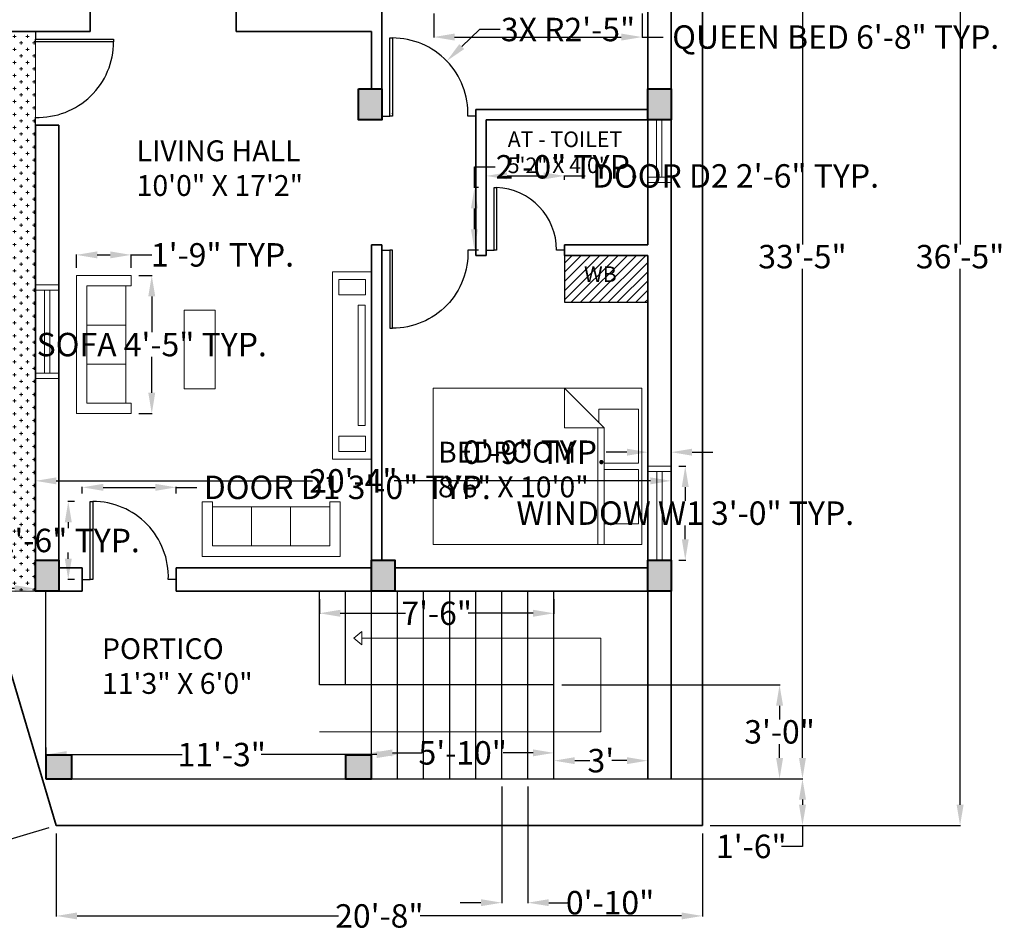
# Model space of a CAD drawing. Units: inches. Extents: x 411 to 983, y 289 to 833.
# Tile 2 of 3: x 605 to 983, y 289 to 639. Entities that reach past the tile are written whole.
import ezdxf

# ---------------------------------------------------------------- set-up
doc = ezdxf.new("R2010")
doc.units = ezdxf.units.IN
doc.header["$MEASUREMENT"] = 0
for name, color, linetype, lineweight in [('A-ANNO-DIMS', 2, 'Continuous', 18), ('A-ANNO-SYMB', 253, 'Continuous', 18), ('A-ANNO-TEXT', 7, 'Continuous', 18), ('A-AREA-IDEN', 7, 'Continuous', 25), ('A-COLS', 18, 'Continuous', 40), ('A-DOOR', 4, 'Continuous', 25), ('A-FLOR-CASE', 2, 'Continuous', 25), ('A-FLOR-OTLN', 4, 'Continuous', 30), ('A-FLOR-PATT', 3, 'Continuous', 13), ('A-FLOR-STRS', 4, 'Continuous', 25), ('A-FURN', 8, 'Continuous', 18), ('A-GLAZ', 4, 'Continuous', 18), ('A-WALL', 4, 'Continuous', 35), ('C-PROP', 4, 'Continuous', 35), ('L-PLNT', 4, 'Continuous', 18), ('L-PLNT-PATT', 3, 'Continuous', 13)]:
    doc.layers.add(name, color=color, linetype=linetype, lineweight=lineweight)
doc.layers.add('A-COLS-PATT', color=244, linetype='Continuous', lineweight=13, true_color=0x991b1e)
doc.styles.get("Standard").update_dxf_attribs({"font": 'arial.ttf'})
doc.dimstyles.get("Standard").update_dxf_attribs({"dimtxt": 9, "dimasz": 8, "dimexe": 0.18, "dimexo": 3, "dimgap": 0.09, "dimtad": 0, "dimtih": 1, "dimtoh": 1, "dimdec": 0, "dimzin": 0, "dimdsep": 46, "dimlunit": 3, "dimtxsty": 'Standard', "dimcen": 0.09, "dimadec": 0, "dimazin": 0, "dimtfac": 1, "dimtdec": 0, "dimtofl": 0, "dimtmove": 0, "dimatfit": 3, "dimfxl": 1, "dimtolj": 1, "dimtzin": 0, "dimarcsym": 0})

# ---------------------------------------------------------------- blocks, each defined once
blk = doc.blocks.new('*D7')
at = {"layer": 'A-ANNO-DIMS', "color": 0, "lineweight": -2, "transparency": 16777216}
for p, q in [((619.14, 326.4), (619.14, 294.53)), ((867.14, 326.4), (867.14, 294.53)), ((627.14, 294.71), (727.52, 294.71)), ((859.14, 294.71), (758.77, 294.71))]:
    blk.add_line(p, q, dxfattribs=at)
at = {"layer": 'A-ANNO-DIMS', "color": 0, "transparency": 16777216}
for points in [[(627.14, 296.04), (627.14, 293.37), (619.14, 294.71)], [(859.14, 296.04), (859.14, 293.37), (867.14, 294.71)]]:
    blk.add_solid(points, dxfattribs=at)
at = {"layer": 'Defpoints', "color": 0, "transparency": 16777216}
for p in [(619.14, 329.4), (867.14, 329.4), (867.14, 294.71)]:
    blk.add_point(p, dxfattribs=at)
at = {"layer": 'A-ANNO-DIMS', "color": 0, "transparency": 16777216, "insert": (743.14, 294.71), "char_height": 9, "attachment_point": 5}
blk.add_mtext('\\A1;20\'-8"', dxfattribs=at)
blk = doc.blocks.new('*D8')
at = {"layer": 'A-ANNO-DIMS', "color": 0, "lineweight": -2, "transparency": 16777216}
for p, q in [((870.14, 347.4), (905.71, 347.4)), ((905.53, 339.4), (905.53, 337.4)), ((870.14, 329.4), (905.71, 329.4)), ((905.53, 329.4), (905.53, 321.4)), ((905.53, 321.4), (897.53, 321.4))]:
    blk.add_line(p, q, dxfattribs=at)
at = {"layer": 'A-ANNO-DIMS', "color": 0, "transparency": 16777216}
for points in [[(904.2, 339.4), (906.87, 339.4), (905.53, 347.4)], [(904.2, 337.4), (906.87, 337.4), (905.53, 329.4)]]:
    blk.add_solid(points, dxfattribs=at)
at = {"layer": 'Defpoints', "color": 0, "transparency": 16777216}
for p in [(867.14, 347.4), (867.14, 329.4), (905.53, 329.4)]:
    blk.add_point(p, dxfattribs=at)
at = {"layer": 'A-ANNO-DIMS', "color": 0, "transparency": 16777216, "insert": (885.9, 321.4), "char_height": 9, "attachment_point": 5}
blk.add_mtext('\\A1;1\'-6"', dxfattribs=at)
blk = doc.blocks.new('*D10')
at = {"layer": 'A-ANNO-DIMS', "color": 0, "lineweight": -2, "transparency": 16777216}
for p, q in [((870.14, 748.4), (905.71, 748.4)), ((905.53, 740.4), (905.53, 552.59)), ((905.53, 355.4), (905.53, 543.21)), ((870.14, 347.4), (905.71, 347.4))]:
    blk.add_line(p, q, dxfattribs=at)
at = {"layer": 'A-ANNO-DIMS', "color": 0, "transparency": 16777216}
for points in [[(904.2, 740.4), (906.87, 740.4), (905.53, 748.4)], [(904.2, 355.4), (906.87, 355.4), (905.53, 347.4)]]:
    blk.add_solid(points, dxfattribs=at)
at = {"layer": 'Defpoints', "color": 0, "transparency": 16777216}
for p in [(867.14, 748.4), (867.14, 347.4), (905.53, 347.4)]:
    blk.add_point(p, dxfattribs=at)
at = {"layer": 'A-ANNO-DIMS', "color": 0, "transparency": 16777216, "insert": (905.53, 547.9), "char_height": 9, "attachment_point": 5}
blk.add_mtext('\\A1;33\'-5"', dxfattribs=at)
blk = doc.blocks.new('*D11')
at = {"layer": 'A-ANNO-DIMS', "color": 0, "lineweight": -2, "transparency": 16777216}
for p, q in [((870.14, 766.4), (966.2, 766.4)), ((966.02, 758.4), (966.02, 552.59)), ((966.02, 337.4), (966.02, 543.21)), ((870.14, 329.4), (966.2, 329.4))]:
    blk.add_line(p, q, dxfattribs=at)
at = {"layer": 'A-ANNO-DIMS', "color": 0, "transparency": 16777216}
for points in [[(964.69, 758.4), (967.36, 758.4), (966.02, 766.4)], [(964.69, 337.4), (967.36, 337.4), (966.02, 329.4)]]:
    blk.add_solid(points, dxfattribs=at)
at = {"layer": 'Defpoints', "color": 0, "transparency": 16777216}
for p in [(867.14, 766.4), (966.02, 766.4), (867.14, 329.4)]:
    blk.add_point(p, dxfattribs=at)
at = {"layer": 'A-ANNO-DIMS', "color": 0, "transparency": 16777216, "insert": (966.02, 547.9), "char_height": 9, "attachment_point": 5}
blk.add_mtext('\\A1;36\'-5"', dxfattribs=at)
blk = doc.blocks.new('*D16')
at = {"layer": 'A-ANNO-DIMS', "color": 0, "lineweight": -2, "transparency": 16777216}
for p, q in [((486.27, 765.55), (411.34, 743.26)), ((413.79, 735.64), (475.12, 529.5)), ((539.23, 313.98), (477.91, 520.12)), ((616.27, 328.55), (541.34, 306.26))]:
    blk.add_line(p, q, dxfattribs=at)
at = {"layer": 'A-ANNO-DIMS', "color": 0, "transparency": 16777216}
for points in [[(415.07, 736.02), (412.52, 735.26), (411.51, 743.31)], [(540.51, 314.36), (537.95, 313.6), (541.51, 306.31)]]:
    blk.add_solid(points, dxfattribs=at)
at = {"layer": 'Defpoints', "color": 0, "transparency": 16777216}
for p in [(489.14, 766.4), (411.51, 743.31), (619.14, 329.4)]:
    blk.add_point(p, dxfattribs=at)
at = {"layer": 'A-ANNO-DIMS', "color": 0, "transparency": 16777216, "insert": (476.51, 524.81), "char_height": 9, "attachment_point": 5}
blk.add_mtext("\\A1;38'", dxfattribs=at)
blk = doc.blocks.new('*D18')
at = {"layer": 'A-ANNO-DIMS', "color": 0, "lineweight": -2, "transparency": 16777216}
for p, q in [((592.37, 420.4), (584.37, 420.4)), ((592.37, 422.4), (592.37, 420.58)), ((603.14, 420.4), (600.37, 420.4)), ((611.14, 422.4), (611.14, 420.58))]:
    blk.add_line(p, q, dxfattribs=at)
at = {"layer": 'A-ANNO-DIMS', "color": 0, "transparency": 16777216}
for points in [[(600.37, 421.73), (600.37, 419.06), (592.37, 420.4)], [(603.14, 421.73), (603.14, 419.06), (611.14, 420.4)]]:
    blk.add_solid(points, dxfattribs=at)
at = {"layer": 'Defpoints', "color": 0, "transparency": 16777216}
for p in [(592.37, 420.4), (592.37, 419.4), (611.14, 419.4)]:
    blk.add_point(p, dxfattribs=at)
at = {"layer": 'A-ANNO-DIMS', "color": 0, "transparency": 16777216, "insert": (572.74, 420.4), "char_height": 9, "attachment_point": 5}
blk.add_mtext('\\A1;1\'-7"', dxfattribs=at)
blk = doc.blocks.new('*D19')
at = {"layer": 'A-ANNO-DIMS', "color": 0, "lineweight": -2, "transparency": 16777216}
for p, q in [((611.14, 434.4), (611.14, 461.98)), ((619.14, 461.8), (717.52, 461.8)), ((847.14, 461.8), (748.77, 461.8)), ((855.14, 434.4), (855.14, 461.98))]:
    blk.add_line(p, q, dxfattribs=at)
at = {"layer": 'A-ANNO-DIMS', "color": 0, "transparency": 16777216}
for points in [[(619.14, 463.13), (619.14, 460.47), (611.14, 461.8)], [(847.14, 463.13), (847.14, 460.47), (855.14, 461.8)]]:
    blk.add_solid(points, dxfattribs=at)
at = {"layer": 'Defpoints', "color": 0, "transparency": 16777216}
for p in [(855.14, 461.8), (611.14, 431.4), (855.14, 431.4)]:
    blk.add_point(p, dxfattribs=at)
at = {"layer": 'A-ANNO-DIMS', "color": 0, "transparency": 16777216, "insert": (733.14, 461.8), "char_height": 9, "width": 31.0703, "attachment_point": 5}
blk.add_mtext('\\A1;20\'-4"', dxfattribs=at)
blk = doc.blocks.new('*D20')
at = {"layer": 'A-ANNO-DIMS', "color": 0, "lineweight": -2, "transparency": 16777216}
for p, q in [((810.14, 350.4), (810.14, 354.52)), ((818.14, 354.34), (823.92, 354.34)), ((838.14, 354.34), (832.37, 354.34)), ((846.14, 350.4), (846.14, 354.52))]:
    blk.add_line(p, q, dxfattribs=at)
at = {"layer": 'A-ANNO-DIMS', "color": 0, "transparency": 16777216}
for points in [[(818.14, 355.67), (818.14, 353), (810.14, 354.34)], [(838.14, 355.67), (838.14, 353), (846.14, 354.34)]]:
    blk.add_solid(points, dxfattribs=at)
at = {"layer": 'Defpoints', "color": 0, "transparency": 16777216}
for p in [(846.14, 354.34), (810.14, 347.4), (846.14, 347.4)]:
    blk.add_point(p, dxfattribs=at)
at = {"layer": 'A-ANNO-DIMS', "color": 0, "transparency": 16777216, "insert": (828.14, 354.34), "char_height": 9, "attachment_point": 5}
blk.add_mtext("\\A1;3'", dxfattribs=at)
blk = doc.blocks.new('*D21')
at = {"layer": 'A-ANNO-DIMS', "color": 0, "lineweight": -2, "transparency": 16777216}
for p, q in [((740.14, 350.4), (740.14, 357.51)), ((748.14, 357.33), (759.6, 357.33)), ((802.14, 357.33), (790.69, 357.33)), ((810.14, 350.4), (810.14, 357.51))]:
    blk.add_line(p, q, dxfattribs=at)
at = {"layer": 'A-ANNO-DIMS', "color": 0, "transparency": 16777216}
for points in [[(748.14, 358.66), (748.14, 356), (740.14, 357.33)], [(802.14, 358.66), (802.14, 356), (810.14, 357.33)]]:
    blk.add_solid(points, dxfattribs=at)
at = {"layer": 'Defpoints', "color": 0, "transparency": 16777216}
for p in [(740.14, 357.33), (740.14, 347.4), (810.14, 347.4)]:
    blk.add_point(p, dxfattribs=at)
at = {"layer": 'A-ANNO-DIMS', "color": 0, "transparency": 16777216, "insert": (775.14, 357.33), "char_height": 9, "attachment_point": 5}
blk.add_mtext('\\A1;5\'-10"', dxfattribs=at)
blk = doc.blocks.new('*D22')
at = {"layer": 'A-ANNO-DIMS', "color": 0, "lineweight": -2, "transparency": 16777216}
for p, q in [((720.14, 416.4), (720.14, 410.76)), ((810.14, 416.4), (810.14, 410.76)), ((728.14, 410.94), (753.13, 410.94)), ((802.14, 410.94), (777.16, 410.94))]:
    blk.add_line(p, q, dxfattribs=at)
at = {"layer": 'A-ANNO-DIMS', "color": 0, "transparency": 16777216}
for points in [[(728.14, 412.28), (728.14, 409.61), (720.14, 410.94)], [(802.14, 412.28), (802.14, 409.61), (810.14, 410.94)]]:
    blk.add_solid(points, dxfattribs=at)
at = {"layer": 'Defpoints', "color": 0, "transparency": 16777216}
for p in [(720.14, 419.4), (810.14, 419.4), (810.14, 410.94)]:
    blk.add_point(p, dxfattribs=at)
at = {"layer": 'A-ANNO-DIMS', "color": 0, "transparency": 16777216, "insert": (765.14, 410.94), "char_height": 9, "attachment_point": 5}
blk.add_mtext('\\A1;7\'-6"', dxfattribs=at)
blk = doc.blocks.new('*D23')
at = {"layer": 'A-ANNO-DIMS', "color": 0, "lineweight": -2, "transparency": 16777216}
for p, q in [((615.14, 359.4), (615.14, 356.85)), ((623.14, 356.67), (667.52, 356.67)), ((742.14, 356.67), (697.77, 356.67)), ((750.14, 354.33), (750.14, 356.49))]:
    blk.add_line(p, q, dxfattribs=at)
at = {"layer": 'A-ANNO-DIMS', "color": 0, "transparency": 16777216}
for points in [[(623.14, 358.01), (623.14, 355.34), (615.14, 356.67)], [(742.14, 358.01), (742.14, 355.34), (750.14, 356.67)]]:
    blk.add_solid(points, dxfattribs=at)
at = {"layer": 'Defpoints', "color": 0, "transparency": 16777216}
for p in [(615.14, 356.4), (750.14, 357.33), (750.14, 356.67)]:
    blk.add_point(p, dxfattribs=at)
at = {"layer": 'A-ANNO-DIMS', "color": 0, "transparency": 16777216, "insert": (682.64, 356.67), "char_height": 9, "attachment_point": 5}
blk.add_mtext('\\A1;11\'-3"', dxfattribs=at)
blk = doc.blocks.new('BED-QUEEN-60X80')
for p, q in [((0, 60), (0, 0)), ((80, 60), (0, 60)), ((50.4, 60), (65.6, 44.8)), ((50.4, 44.8), (50.4, 60)), ((80, 0), (80, 60)), ((63.6, 52), (63.6, 46.8)), ((78.8, 52), (63.6, 52)), ((78.8, 31.2), (78.8, 52)), ((65.6, 44.8), (50.4, 44.8)), ((63.2, 44.8), (63.2, 0)), ((65.6, 0), (65.6, 44.8)), ((65.6, 31.2), (78.8, 31.2)), ((78.8, 28.8), (65.6, 28.8)), ((78.8, 8), (78.8, 28.8)), ((65.6, 8), (78.8, 8)), ((0, 0), (80, 0))]:
    blk.add_line(p, q)
blk = doc.blocks.new('SOFA-3SEAT-53')
for p, q in [((4, 21), (0, 21)), ((0, 21), (0, 19)), ((0, 4), (0, 19)), ((4, 19), (4, 21)), ((4, 4), (4, 19)), ((4, 19), (49, 19)), ((19, 4), (19, 19)), ((34, 19), (34, 4)), ((49, 19), (49, 21)), ((49, 21), (53, 21)), ((49, 19), (49, 4)), ((53, 21), (53, 19)), ((53, 19), (53, 4)), ((0, 4), (0, 0)), ((49, 4), (4, 4)), ((53, 4), (53, 0)), ((0, 0), (4, 0)), ((49, 0), (4, 0)), ((53, 0), (49, 0))]:
    blk.add_line(p, q)
blk = doc.blocks.new('DOOR-SWING-36')
for p, q in [((3, 0), (3, 30)), ((3, 30), (4, 30)), ((4, 30), (4, 0)), ((0, 0), (3, 0)), ((4, 0), (3, 0)), ((36, 0), (33, 0))]:
    blk.add_line(p, q)
blk.add_arc((4, 0.98), 29.02, 358.058, 90)
blk = doc.blocks.new('DOOR-SWING-30')
for p, q in [((3, 0), (3, 24)), ((3, 24), (4, 24)), ((4, 24), (4, 0)), ((0, 0), (3, 0)), ((4, 0), (3, 0)), ((30, 0), (27, 0))]:
    blk.add_line(p, q)
blk.add_arc((3.13, 0.15), 23.87, 359.6418, 87.9204)
blk = doc.blocks.new('WIN-36-POST')
for p, q in [((34, 0), (34, 9)), ((36, 0), (36, 9)), ((34, 5.5), (0, 5.5)), ((34, 3.5), (0, 3.5))]:
    blk.add_line(p, q)
blk = doc.blocks.new('WIN-24-POST')
for p, q in [((0, 9), (0, 0)), ((2, 9), (2, 0)), ((24, 5.5), (2, 5.5)), ((24, 3.5), (2, 3.5))]:
    blk.add_line(p, q)
blk = doc.blocks.new('*D30')
at = {"layer": 'A-ANNO-DIMS', "color": 0, "lineweight": -2, "transparency": 16777216}
for p, q in [((629.14, 456.9), (629.14, 459.48)), ((637.14, 459.3), (657.14, 459.3)), ((665.14, 456.9), (665.14, 459.48)), ((665.14, 459.3), (673.14, 459.3))]:
    blk.add_line(p, q, dxfattribs=at)
at = {"layer": 'A-ANNO-DIMS', "color": 0, "transparency": 16777216}
for points in [[(637.14, 460.64), (637.14, 457.97), (629.14, 459.3)], [(657.14, 460.64), (657.14, 457.97), (665.14, 459.3)]]:
    blk.add_solid(points, dxfattribs=at)
at = {"layer": 'Defpoints', "color": 0, "transparency": 16777216}
for p in [(665.14, 459.3), (629.14, 453.9), (665.14, 453.9)]:
    blk.add_point(p, dxfattribs=at)
at = {"layer": 'A-ANNO-DIMS', "color": 0, "transparency": 16777216, "insert": (730.83, 459.3), "char_height": 9, "attachment_point": 5}
blk.add_mtext('\\A1;DOOR D1 3\'-0" TYP.', dxfattribs=at)
blk = doc.blocks.new('*D31')
at = {"layer": 'A-ANNO-DIMS', "color": 0, "lineweight": -2, "transparency": 16777216}
for p, q in [((626.14, 453.9), (623.56, 453.9)), ((623.74, 445.9), (623.74, 443.59)), ((623.74, 431.9), (623.74, 434.22)), ((626.14, 423.9), (623.56, 423.9))]:
    blk.add_line(p, q, dxfattribs=at)
at = {"layer": 'A-ANNO-DIMS', "color": 0, "transparency": 16777216}
for points in [[(622.41, 445.9), (625.08, 445.9), (623.74, 453.9)], [(622.41, 431.9), (625.08, 431.9), (623.74, 423.9)]]:
    blk.add_solid(points, dxfattribs=at)
at = {"layer": 'Defpoints', "color": 0, "transparency": 16777216}
for p in [(623.74, 453.9), (629.14, 453.9), (629.14, 423.9)]:
    blk.add_point(p, dxfattribs=at)
at = {"layer": 'A-ANNO-DIMS', "color": 0, "transparency": 16777216, "insert": (623.74, 438.9), "char_height": 9, "attachment_point": 5}
blk.add_mtext('\\A1;2\'-6" TYP.', dxfattribs=at)
blk = doc.blocks.new('*D32')
at = {"layer": 'A-ANNO-DIMS', "color": 0, "lineweight": -2, "transparency": 16777216}
for p, q in [((784.14, 577.4), (784.14, 579.08)), ((792.14, 578.9), (806.14, 578.9)), ((814.14, 577.4), (814.14, 579.08)), ((814.14, 578.9), (822.14, 578.9))]:
    blk.add_line(p, q, dxfattribs=at)
at = {"layer": 'A-ANNO-DIMS', "color": 0, "transparency": 16777216}
for points in [[(792.14, 580.24), (792.14, 577.57), (784.14, 578.9)], [(806.14, 580.24), (806.14, 577.57), (814.14, 578.9)]]:
    blk.add_solid(points, dxfattribs=at)
at = {"layer": 'Defpoints', "color": 0, "transparency": 16777216}
for p in [(814.14, 578.9), (784.14, 574.4), (814.14, 574.4)]:
    blk.add_point(p, dxfattribs=at)
at = {"layer": 'A-ANNO-DIMS', "color": 0, "transparency": 16777216, "insert": (879.83, 578.9), "char_height": 9, "attachment_point": 5}
blk.add_mtext('\\A1;DOOR D2 2\'-6" TYP.', dxfattribs=at)
blk = doc.blocks.new('*D33')
at = {"layer": 'A-ANNO-DIMS', "color": 0, "lineweight": -2, "transparency": 16777216}
for p, q in [((779.64, 574.4), (779.64, 582.4)), ((779.64, 582.4), (787.64, 582.4)), ((781.14, 574.4), (779.46, 574.4)), ((779.64, 558.4), (779.64, 566.4)), ((781.14, 550.4), (779.46, 550.4))]:
    blk.add_line(p, q, dxfattribs=at)
at = {"layer": 'A-ANNO-DIMS', "color": 0, "transparency": 16777216}
for points in [[(778.31, 566.4), (780.98, 566.4), (779.64, 574.4)], [(778.31, 558.4), (780.98, 558.4), (779.64, 550.4)]]:
    blk.add_solid(points, dxfattribs=at)
at = {"layer": 'Defpoints', "color": 0, "transparency": 16777216}
for p in [(779.64, 574.4), (784.14, 574.4), (784.14, 550.4)]:
    blk.add_point(p, dxfattribs=at)
at = {"layer": 'A-ANNO-DIMS', "color": 0, "transparency": 16777216, "insert": (815.24, 582.4), "char_height": 9, "attachment_point": 5}
blk.add_mtext('\\A1;2\'-0" TYP.', dxfattribs=at)
blk = doc.blocks.new('*D34')
at = {"layer": 'A-ANNO-DIMS', "color": 0, "lineweight": -2, "transparency": 16777216}
for p, q in [((858.14, 467.4), (860.72, 467.4)), ((860.54, 459.4), (860.54, 454.15)), ((860.54, 439.4), (860.54, 444.65)), ((858.14, 431.4), (860.72, 431.4))]:
    blk.add_line(p, q, dxfattribs=at)
at = {"layer": 'A-ANNO-DIMS', "color": 0, "transparency": 16777216}
for points in [[(859.21, 459.4), (861.88, 459.4), (860.54, 467.4)], [(859.21, 439.4), (861.88, 439.4), (860.54, 431.4)]]:
    blk.add_solid(points, dxfattribs=at)
at = {"layer": 'Defpoints', "color": 0, "transparency": 16777216}
for p in [(855.14, 467.4), (860.54, 467.4), (855.14, 431.4)]:
    blk.add_point(p, dxfattribs=at)
at = {"layer": 'A-ANNO-DIMS', "color": 0, "transparency": 16777216, "insert": (860.54, 449.4), "char_height": 9, "attachment_point": 5}
blk.add_mtext('\\A1;WINDOW W1 3\'-0" TYP.', dxfattribs=at)
blk = doc.blocks.new('*D35')
at = {"layer": 'A-ANNO-DIMS', "color": 0, "lineweight": -2, "transparency": 16777216}
for p, q in [((838.14, 472.8), (830.14, 472.8)), ((846.14, 470.4), (846.14, 472.98)), ((855.14, 470.4), (855.14, 472.98)), ((863.14, 472.8), (871.14, 472.8))]:
    blk.add_line(p, q, dxfattribs=at)
at = {"layer": 'A-ANNO-DIMS', "color": 0, "transparency": 16777216}
for points in [[(838.14, 474.14), (838.14, 471.47), (846.14, 472.8)], [(863.14, 474.14), (863.14, 471.47), (855.14, 472.8)]]:
    blk.add_solid(points, dxfattribs=at)
at = {"layer": 'Defpoints', "color": 0, "transparency": 16777216}
for p in [(846.14, 472.8), (846.14, 467.4), (855.14, 467.4)]:
    blk.add_point(p, dxfattribs=at)
at = {"layer": 'A-ANNO-DIMS', "color": 0, "transparency": 16777216, "insert": (802.62, 472.8), "char_height": 9, "attachment_point": 5}
blk.add_mtext('\\A1;0\'-9" TYP.', dxfattribs=at)
blk = doc.blocks.new('*D38')
at = {"layer": 'A-ANNO-DIMS', "color": 0, "lineweight": -2, "transparency": 16777216}
for p, q in [((650.84, 540.63), (655.97, 540.63)), ((655.79, 532.63), (655.79, 518.88)), ((655.79, 495.63), (655.79, 509.38)), ((650.84, 487.63), (655.97, 487.63))]:
    blk.add_line(p, q, dxfattribs=at)
at = {"layer": 'A-ANNO-DIMS', "color": 0, "transparency": 16777216}
for points in [[(654.45, 532.63), (657.12, 532.63), (655.79, 540.63)], [(654.45, 495.63), (657.12, 495.63), (655.79, 487.63)]]:
    blk.add_solid(points, dxfattribs=at)
at = {"layer": 'Defpoints', "color": 0, "transparency": 16777216}
for p in [(647.84, 540.63), (647.84, 487.63), (655.79, 487.63)]:
    blk.add_point(p, dxfattribs=at)
at = {"layer": 'A-ANNO-DIMS', "color": 0, "transparency": 16777216, "insert": (655.79, 514.13), "char_height": 9, "attachment_point": 5}
blk.add_mtext('\\A1;SOFA 4\'-5" TYP.', dxfattribs=at)
blk = doc.blocks.new('*D39')
at = {"layer": 'A-ANNO-DIMS', "color": 0, "lineweight": -2, "transparency": 16777216}
for p, q in [((626.84, 543.63), (626.84, 548.76)), ((634.84, 548.58), (639.84, 548.58)), ((647.84, 543.63), (647.84, 548.76)), ((647.84, 548.58), (655.84, 548.58))]:
    blk.add_line(p, q, dxfattribs=at)
at = {"layer": 'A-ANNO-DIMS', "color": 0, "transparency": 16777216}
for points in [[(634.84, 549.91), (634.84, 547.25), (626.84, 548.58)], [(639.84, 549.91), (639.84, 547.25), (647.84, 548.58)]]:
    blk.add_solid(points, dxfattribs=at)
at = {"layer": 'Defpoints', "color": 0, "transparency": 16777216}
for p in [(647.84, 548.58), (626.84, 540.63), (647.84, 540.63)]:
    blk.add_point(p, dxfattribs=at)
at = {"layer": 'A-ANNO-DIMS', "color": 0, "transparency": 16777216, "insert": (682.93, 548.58), "char_height": 9, "attachment_point": 5}
blk.add_mtext('\\A1;1\'-9" TYP.', dxfattribs=at)
blk = doc.blocks.new('*D40')
at = {"layer": 'A-ANNO-DIMS', "color": 0, "lineweight": -2, "transparency": 16777216}
for p, q in [((764, 641.23), (764, 632.05)), ((844, 641.23), (844, 632.05)), ((772, 632.23), (836, 632.23)), ((844, 632.23), (852, 632.23))]:
    blk.add_line(p, q, dxfattribs=at)
at = {"layer": 'A-ANNO-DIMS', "color": 0, "transparency": 16777216}
for points in [[(772, 633.56), (772, 630.89), (764, 632.23)], [(836, 633.56), (836, 630.89), (844, 632.23)]]:
    blk.add_solid(points, dxfattribs=at)
at = {"layer": 'Defpoints', "color": 0, "transparency": 16777216}
for p in [(764, 644.23), (844, 644.23), (844, 632.23)]:
    blk.add_point(p, dxfattribs=at)
at = {"layer": 'A-ANNO-DIMS', "color": 0, "transparency": 16777216, "insert": (918.29, 632.23), "char_height": 9, "attachment_point": 5}
blk.add_mtext('\\A1;QUEEN BED 6\'-8" TYP.', dxfattribs=at)
blk = doc.blocks.new('*D43')
at = {"layer": 'A-ANNO-DIMS', "color": 0, "lineweight": -2, "transparency": 16777216}
for p, q in [((790.14, 344.4), (790.14, 299.62)), ((800.14, 344.4), (800.14, 299.62)), ((782.14, 299.8), (774.14, 299.8)), ((808.14, 299.8), (816.14, 299.8))]:
    blk.add_line(p, q, dxfattribs=at)
at = {"layer": 'A-ANNO-DIMS', "color": 0, "transparency": 16777216}
for points in [[(782.14, 301.14), (782.14, 298.47), (790.14, 299.8)], [(808.14, 301.14), (808.14, 298.47), (800.14, 299.8)]]:
    blk.add_solid(points, dxfattribs=at)
at = {"layer": 'Defpoints', "color": 0, "transparency": 16777216}
for p in [(790.14, 347.4), (800.14, 347.4), (800.14, 299.8)]:
    blk.add_point(p, dxfattribs=at)
at = {"layer": 'A-ANNO-DIMS', "color": 0, "transparency": 16777216, "insert": (831.69, 299.8), "char_height": 9, "attachment_point": 5}
blk.add_mtext('\\A1;0\'-10"', dxfattribs=at)
blk = doc.blocks.new('*D46')
at = {"layer": 'A-ANNO-DIMS', "color": 0, "lineweight": -2, "transparency": 16777216}
for p, q in [((813.14, 383.4), (896.92, 383.4)), ((896.74, 375.4), (896.74, 370.09)), ((896.74, 355.4), (896.74, 360.71)), ((813.14, 347.4), (896.92, 347.4))]:
    blk.add_line(p, q, dxfattribs=at)
at = {"layer": 'A-ANNO-DIMS', "color": 0, "transparency": 16777216}
for points in [[(895.41, 375.4), (898.08, 375.4), (896.74, 383.4)], [(895.41, 355.4), (898.08, 355.4), (896.74, 347.4)]]:
    blk.add_solid(points, dxfattribs=at)
at = {"layer": 'Defpoints', "color": 0, "transparency": 16777216}
for p in [(810.14, 383.4), (896.74, 383.4), (810.14, 347.4)]:
    blk.add_point(p, dxfattribs=at)
at = {"layer": 'A-ANNO-DIMS', "color": 0, "transparency": 16777216, "insert": (896.74, 365.4), "char_height": 9, "attachment_point": 5}
blk.add_mtext('\\A1;3\'-0"', dxfattribs=at)
blk = doc.blocks.new('*D47')
at = {"layer": 'A-ANNO-DIMS', "color": 0, "lineweight": -2, "transparency": 16777216}
for p, q in [((781.52, 635.12), (774.76, 628.58)), ((789.52, 635.12), (781.52, 635.12)), ((748.05, 602.85), (748.23, 602.85)), ((748.14, 602.76), (748.14, 602.94))]:
    blk.add_line(p, q, dxfattribs=at)
at = {"layer": 'A-ANNO-DIMS', "color": 0, "transparency": 16777216}
blk.add_solid([(773.83, 629.54), (775.68, 627.62), (769.01, 623.02)], dxfattribs=at)
at = {"layer": 'Defpoints', "color": 0, "transparency": 16777216}
for p in [(769.01, 623.02), (748.14, 602.85)]:
    blk.add_point(p, dxfattribs=at)
at = {"layer": 'A-ANNO-DIMS', "color": 0, "transparency": 16777216, "insert": (815.55, 635.12), "char_height": 9, "attachment_point": 5}
blk.add_mtext('\\A1;3X R2\'-5"', dxfattribs=at)

msp = doc.modelspace()

# ---------------------------------------------------------------- hatches: boundary and pattern name
at = {"layer": 'A-COLS-PATT'}
h = msp.add_hatch(color=256, dxfattribs=at)
h.dxf.hatch_style = 1
h.paths.add_polyline_path([(625.14, 347.4), (625.14, 356.4), (615.14, 356.4), (615.14, 347.4)])
h.paths.add_polyline_path([(740.14, 347.4), (740.14, 356.4), (730.14, 356.4), (730.14, 347.4)])
h.paths.add_polyline_path([(740.14, 419.4), (749.14, 419.4), (749.14, 431.4), (740.14, 431.4)])
h.paths.add_polyline_path([(611.14, 419.4), (620.14, 419.4), (620.14, 431.4), (611.14, 431.4)])
h.paths.add_polyline_path([(846.14, 419.4), (855.14, 419.4), (855.14, 431.4), (846.14, 431.4)])
h.paths.add_polyline_path([(855.14, 612.4), (846.14, 612.4), (846.14, 600.4), (855.14, 600.4)])
h.paths.add_polyline_path([(744.14, 612.4), (735.14, 612.4), (735.14, 600.4), (744.14, 600.4)])
h.paths.add_polyline_path([(546.14, 634.4), (555.14, 634.4), (555.14, 646.4), (546.14, 646.4)])
h.paths.add_polyline_path([(555.14, 748.4), (546.14, 748.4), (546.14, 736.4), (555.14, 736.4)])
h.paths.add_polyline_path([(744.14, 748.4), (732.14, 748.4), (732.14, 739.4), (744.14, 739.4)])
h.paths.add_polyline_path([(855.14, 748.4), (846.14, 748.4), (846.14, 736.4), (855.14, 736.4)])
at = {"layer": 'A-FLOR-PATT'}
h = msp.add_hatch(dxfattribs=at)
h.set_pattern_fill('ANSI31', color=256, scale=20)
h.paths.add_polyline_path([(846.14, 739.4), (780.14, 739.4), (780.14, 721.4), (846.14, 721.4)])
h.paths.add_polyline_path([(846.14, 548.4), (814.14, 548.4), (814.14, 530.4), (846.14, 530.4)])
h.paths.add_polyline_path([(807.66, 726.4), (824.16, 726.4), (824.16, 738.76), (807.66, 738.76)], flags=24)
h.paths.add_polyline_path([(820.06, 534.9), (836.57, 534.9), (836.57, 547.26), (820.06, 547.26)], flags=24)
at = {"layer": 'L-PLNT-PATT'}
h = msp.add_hatch(dxfattribs=at)
h.set_pattern_fill('CROSS', color=256, scale=10)
h.paths.add_polyline_path([(611.14, 598.4), (611.14, 601.4), (611.14, 634.4), (528.41, 634.4), (592.37, 419.4), (611.14, 419.4), (611.14, 431.4)])
h.paths.add_polyline_path([(552.04, 568.07), (588.33, 568.07), (588.33, 584.55), (552.04, 584.55)], flags=24)

# ---------------------------------------------------------------- linework, layer by layer
at = {"layer": 'A-ANNO-SYMB'}
for p, q in [((733.28, 401.4), (736.35, 403.95)), ((733.28, 401.4), (736.35, 398.85)), ((736.35, 398.85), (736.35, 403.95)), ((828.14, 401.4), (736.35, 401.4)), ((828.14, 365.4), (828.14, 401.4)), ((828.14, 365.4), (720.14, 365.4))]:
    msp.add_line(p, q, dxfattribs=at)
at = {"layer": 'A-COLS'}
for points in [[(735.14, 612.4), (744.14, 612.4), (744.14, 600.4), (735.14, 600.4)], [(846.14, 612.4), (855.14, 612.4), (855.14, 600.4), (846.14, 600.4)], [(611.14, 431.4), (620.14, 431.4), (620.14, 419.4), (611.14, 419.4)], [(740.14, 431.4), (749.14, 431.4), (749.14, 419.4), (740.14, 419.4)], [(846.14, 431.4), (855.14, 431.4), (855.14, 419.4), (846.14, 419.4)], [(615.14, 347.4), (625.14, 347.4), (625.14, 356.4), (615.14, 356.4)], [(730.14, 347.4), (740.14, 347.4), (740.14, 356.4), (730.14, 356.4)]]:
    msp.add_lwpolyline(points, close=True, dxfattribs=at)
at = {"layer": 'A-DOOR'}
for p, q in [((611.14, 634.4), (611.14, 631.4)), ((611.14, 631.4), (641.14, 631.4)), ((611.14, 630.4), (611.14, 631.4)), ((641.14, 631.4), (641.14, 630.4)), ((641.14, 630.4), (611.14, 630.4)), ((611.14, 598.4), (611.14, 601.4))]:
    msp.add_line(p, q, dxfattribs=at)
msp.add_arc((612.13, 630.4), 29.02, 268.058, 0, dxfattribs=at)
at = {"layer": 'A-FLOR-CASE'}
for p, q in [((814.14, 548.4), (814.14, 530.4)), ((814.14, 530.4), (846.14, 530.4))]:
    msp.add_line(p, q, dxfattribs=at)
at = {"layer": 'A-FLOR-OTLN'}
for q in [(615.14, 419.4), (855.14, 347.4)]:
    msp.add_line((615.14, 347.4), q, dxfattribs=at)
at = {"layer": 'A-FLOR-STRS'}
for p, q in [((720.14, 383.4), (720.14, 419.4)), ((730.14, 383.4), (730.14, 419.4)), ((740.14, 347.4), (740.14, 419.4)), ((740.14, 347.4), (740.14, 419.4)), ((750.14, 347.4), (750.14, 419.4)), ((760.14, 347.4), (760.14, 419.4)), ((770.14, 347.4), (770.14, 419.4)), ((780.14, 347.4), (780.14, 419.4)), ((790.14, 347.4), (790.14, 419.4)), ((800.14, 347.4), (800.14, 419.4)), ((810.14, 347.4), (810.14, 419.4)), ((810.14, 383.4), (720.14, 383.4))]:
    msp.add_line(p, q, dxfattribs=at)
at = {"layer": 'A-FURN'}
for p, q in [((740.14, 542.1), (725.14, 542.1)), ((725.14, 542.1), (725.14, 470.1)), ((725.14, 470.1), (740.14, 470.1))]:
    msp.add_line(p, q, dxfattribs=at)
for points in [[(727.58, 539.16), (737.8, 539.16), (737.8, 533.22), (727.58, 533.22)], [(737.69, 482.99), (734.98, 482.99), (734.98, 529.21), (737.69, 529.21)], [(668.21, 497.09), (680.15, 497.09), (680.15, 527.4), (668.21, 527.4)], [(727.58, 478.96), (737.8, 478.96), (737.8, 473.02), (727.58, 473.02)]]:
    msp.add_lwpolyline(points, close=True, dxfattribs=at)
at = {"layer": 'A-GLAZ'}
for p, q in [((620.14, 537.09), (611.14, 537.09)), ((620.14, 535.09), (611.14, 535.09)), ((614.64, 535.09), (614.64, 503.09)), ((616.64, 535.09), (616.64, 503.09)), ((620.14, 503.09), (611.14, 503.09)), ((620.14, 501.09), (611.14, 501.09))]:
    msp.add_line(p, q, dxfattribs=at)
at = {"layer": 'A-WALL'}
for p, q in [((855.14, 347.4), (855.14, 748.4)), ((688.14, 634.4), (688.14, 739.4)), ((846.14, 604.4), (846.14, 739.4)), ((632.14, 634.4), (632.14, 643.4)), ((744.14, 600.4), (744.14, 643.4)), ((611.14, 634.4), (528.41, 634.4)), ((620.14, 634.4), (611.14, 634.4)), ((620.14, 634.4), (632.14, 634.4)), ((740.14, 634.4), (688.14, 634.4)), ((740.14, 612.4), (740.14, 634.4)), ((846.14, 604.4), (780.14, 604.4)), ((780.14, 548.4), (780.14, 604.4)), ((611.14, 598.4), (611.14, 419.4)), ((620.14, 598.4), (611.14, 598.4)), ((620.14, 598.4), (620.14, 428.4)), ((744.14, 600.4), (740.14, 600.4)), ((846.14, 600.4), (784.14, 600.4)), ((784.14, 552.4), (784.14, 600.4)), ((846.14, 552.4), (846.14, 600.4)), ((740.14, 548.4), (740.14, 552.4)), ((744.14, 552.4), (740.14, 552.4)), ((744.14, 548.4), (744.14, 552.4)), ((784.14, 552.4), (784.14, 548.4)), ((846.14, 552.4), (814.14, 552.4)), ((814.14, 552.4), (814.14, 548.4)), ((740.14, 548.4), (740.14, 428.4)), ((744.14, 548.4), (744.14, 431.4)), ((784.14, 548.4), (780.14, 548.4)), ((846.14, 548.4), (814.14, 548.4)), ((846.14, 428.4), (846.14, 548.4)), ((629.14, 428.4), (620.14, 428.4)), ((629.14, 428.4), (629.14, 419.4)), ((740.14, 428.4), (665.14, 428.4)), ((665.14, 428.4), (665.14, 419.4)), ((846.14, 428.4), (749.14, 428.4)), ((629.14, 419.4), (611.14, 419.4)), ((846.14, 419.4), (665.14, 419.4)), ((846.14, 347.4), (846.14, 419.4))]:
    msp.add_line(p, q, dxfattribs=at)
at = {"layer": 'C-PROP'}
for p, q in [((489.14, 766.4), (619.14, 329.4)), ((867.14, 329.4), (867.14, 766.4)), ((619.14, 329.4), (867.14, 329.4))]:
    msp.add_line(p, q, dxfattribs=at)
at = {"layer": 'L-PLNT'}
for p, q in [((611.14, 598.4), (611.14, 634.4)), ((611.14, 419.4), (592.37, 419.4))]:
    msp.add_line(p, q, dxfattribs=at)

# ---------------------------------------------------------------- block references
at = {"layer": 'A-DOOR'}
for name, p in [('DOOR-SWING-36', (744.14, 601.87)), ('DOOR-SWING-30', (784.14, 550.4)), ('DOOR-SWING-36', (629.14, 423.9))]:
    msp.add_blockref(name, p, dxfattribs=at)
at = {"layer": 'A-DOOR', "extrusion": (0, 0, -1), "zscale": -1, "rotation": 180}
msp.add_blockref('DOOR-SWING-36', (-744.14, 550.4), dxfattribs=at)
at = {"layer": 'A-FURN', "rotation": 269.9999999999985}
msp.add_blockref('SOFA-3SEAT-53', (626.84, 540.63), dxfattribs=at)
at = {"layer": 'A-FURN'}
for name, p in [('BED-QUEEN-60X80', (763.83, 437.35)), ('SOFA-3SEAT-53', (675.08, 432.8))]:
    msp.add_blockref(name, p, dxfattribs=at)
at = {"layer": 'A-GLAZ'}
for name, p, rotation in [('WIN-24-POST', (855.05, 576.4), 89.99999999999883), ('WIN-36-POST', (855.14, 431.4), 89.99999999999976)]:
    msp.add_blockref(name, p, dxfattribs=dict(at, rotation=rotation))

# ---------------------------------------------------------------- texts
at = {"layer": 'A-ANNO-TEXT', "insert": (821.67, 544.17), "char_height": 6, "attachment_point": 1}
msp.add_mtext_dynamic_manual_height_columns('WB', width=69.531, gutter_width=1, heights=[0], dxfattribs=at)
at = {"layer": 'A-AREA-IDEN', "attachment_point": 1}
for s, insert, char_height in [('AT - TOILET\\P5\'2" X 4\'0"', (792.4, 595.98), 6), ('LIVING HALL\\P10\'0" X 17\'2"', (649.97, 592.55), 8), ('BEDROOM\\P8\'6" X 10\'0"', (765.65, 476.81), 8), ('PORTICO\\P11\'3" X 6\'0"', (636.68, 401.33), 8)]:
    msp.add_mtext_dynamic_manual_height_columns(s, width=69.531, gutter_width=1, heights=[0], dxfattribs=dict(at, insert=insert, char_height=char_height))

# ---------------------------------------------------------------- dimensions: what is measured, and where the dimension line sits
at = {"layer": 'A-ANNO-DIMS'}
dim = msp.add_aligned_dim(p1=(619.14, 329.4), p2=(489.14, 766.4), distance=80.99, dimstyle='Standard', override={"dimclrd": 0, "dimclre": 0, "dimclrt": 0}, dxfattribs=at)
dim.commit()
dim.dimension.update_dxf_attribs({"geometry": '*D16', "text_midpoint": (476.51, 524.81)})
for base, p1, p2, override, picture, middle in [((966.02, 766.4), (867.14, 329.4), (867.14, 766.4), {"dimclrd": 0, "dimclre": 0, "dimclrt": 0}, '*D11', (966.02, 547.9)), ((905.53, 347.4), (867.14, 748.4), (867.14, 347.4), {"dimclrd": 0, "dimclre": 0, "dimclrt": 0}, '*D10', (905.53, 547.9)), ((896.74, 383.4), (810.14, 347.4), (810.14, 383.4), {"dimdec": 1, "dimlfac": 1, "dimrnd": 0, "dimzin": 1, "dimdsep": 46, "dimlunit": 4, "dimfrac": 2}, '*D46', (896.74, 365.4)), ((905.53, 329.4), (867.14, 347.4), (867.14, 329.4), {"dimclrd": 0, "dimclre": 0, "dimclrt": 0}, '*D8', (885.9, 321.4))]:
    dim = msp.add_linear_dim(base=base, p1=p1, p2=p2, angle=90, dimstyle='Standard', override=override, dxfattribs=at)
    dim.commit()
    dim.dimension.update_dxf_attribs({"geometry": picture, "text_midpoint": middle})
for base, p1, p2, text, picture, middle in [((844, 632.23), (764, 644.23), (844, 644.23), 'QUEEN BED <> TYP.', '*D40', (918.29, 632.23)), ((814.14, 578.9), (784.14, 574.4), (814.14, 574.4), 'DOOR D2 <> TYP.', '*D32', (879.83, 578.9)), ((647.84, 548.58), (626.84, 540.63), (647.84, 540.63), '<> TYP.', '*D39', (682.93, 548.58)), ((665.14, 459.3), (629.14, 453.9), (665.14, 453.9), 'DOOR D1 <> TYP.', '*D30', (730.83, 459.3))]:
    dim = msp.add_linear_dim(base=base, p1=p1, p2=p2, text=text, dimstyle='Standard', override={"dimdec": 1, "dimlfac": 1, "dimrnd": 0, "dimzin": 1, "dimdsep": 46, "dimlunit": 4, "dimfrac": 2}, dxfattribs=at)
    dim.commit()
    dim.dimension.update_dxf_attribs({"geometry": picture, "text_midpoint": middle})
dim = msp.add_radius_dim(center=(748.14, 602.85), mpoint=(769.01, 623.02), text='3X <>', dimstyle='Standard', override={"dimdec": 1, "dimlfac": 1, "dimrnd": 0, "dimzin": 1, "dimdsep": 46, "dimlunit": 4, "dimfrac": 2}, dxfattribs=at)
dim.commit()
dim.dimension.update_dxf_attribs({"geometry": '*D47', "text_midpoint": (815.55, 635.12), "dimtype": 164})
for base, p1, p2, angle, text, picture, middle in [((779.64, 574.4), (784.14, 550.4), (784.14, 574.4), 90, '<> TYP.', '*D33', (815.24, 582.4)), ((655.79, 487.63), (647.84, 540.63), (647.84, 487.63), 270, 'SOFA <> TYP.', '*D38', (655.79, 514.13)), ((846.14, 472.8), (855.14, 467.4), (846.14, 467.4), 180, '<> TYP.', '*D35', (802.62, 472.8)), ((860.54, 467.4), (855.14, 431.4), (855.14, 467.4), 90, 'WINDOW W1 <> TYP.', '*D34', (860.54, 449.4)), ((623.74, 453.9), (629.14, 423.9), (629.14, 453.9), 90, '<> TYP.', '*D31', (623.74, 438.9))]:
    dim = msp.add_linear_dim(base=base, p1=p1, p2=p2, angle=angle, text=text, dimstyle='Standard', override={"dimdec": 1, "dimlfac": 1, "dimrnd": 0, "dimzin": 1, "dimdsep": 46, "dimlunit": 4, "dimfrac": 2}, dxfattribs=at)
    dim.commit()
    dim.dimension.update_dxf_attribs({"geometry": picture, "text_midpoint": middle})
for base, p1, p2, override, picture, middle in [((855.14, 461.8), (611.14, 431.4), (855.14, 431.4), {"dimclrd": 0, "dimclre": 0, "dimclrt": 0}, '*D19', (733.14, 461.8)), ((592.37, 420.4), (611.14, 419.4), (592.37, 419.4), {"dimclrd": 0, "dimclre": 0, "dimclrt": 0}, '*D18', (572.74, 420.4)), ((810.14, 410.94), (720.14, 419.4), (810.14, 419.4), {"dimclrd": 0, "dimclre": 0, "dimclrt": 0}, '*D22', (765.14, 410.94)), ((740.14, 357.33), (810.14, 347.4), (740.14, 347.4), {"dimclrd": 0, "dimclre": 0, "dimclrt": 0}, '*D21', (775.14, 357.33)), ((750.14, 356.67), (615.14, 356.4), (750.14, 357.33), {"dimclrd": 0, "dimclre": 0, "dimclrt": 0}, '*D23', (682.64, 356.67)), ((846.14, 354.34), (810.14, 347.4), (846.14, 347.4), {"dimclrd": 0, "dimclre": 0, "dimclrt": 0}, '*D20', (828.14, 354.34)), ((800.14, 299.8), (790.14, 347.4), (800.14, 347.4), {"dimdec": 1, "dimlfac": 1, "dimrnd": 0, "dimzin": 1, "dimdsep": 46, "dimlunit": 4, "dimfrac": 2}, '*D43', (831.69, 299.8)), ((867.14, 294.71), (619.14, 329.4), (867.14, 329.4), {"dimclrd": 0, "dimclre": 0, "dimclrt": 0}, '*D7', (743.14, 294.71))]:
    dim = msp.add_linear_dim(base=base, p1=p1, p2=p2, dimstyle='Standard', override=override, dxfattribs=at)
    dim.commit()
    dim.dimension.update_dxf_attribs({"geometry": picture, "text_midpoint": middle})

doc.saveas('drawing.dxf')
